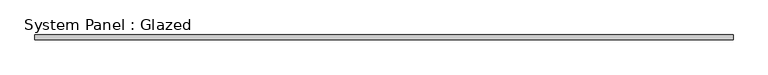
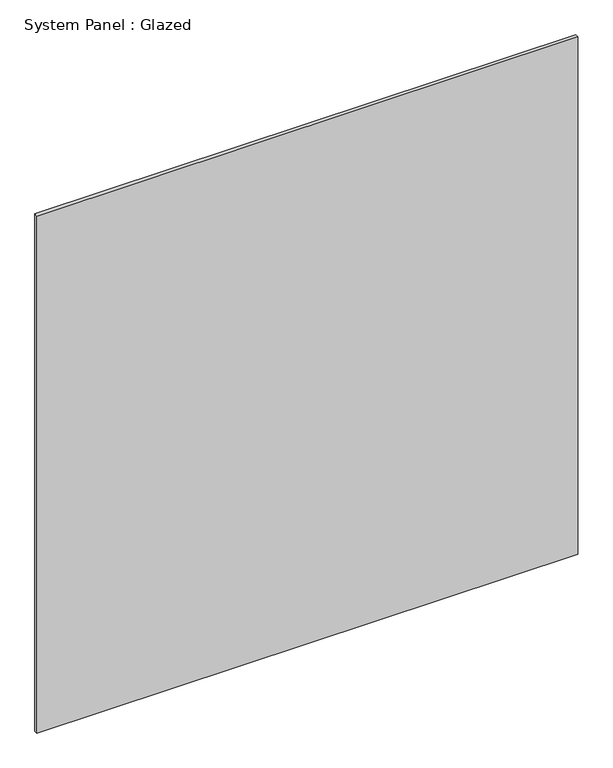
"""IFC4 building model written with IfcOpenShell, lengths in millimetres: plate geometry, System Panel : Glazed."""

from ifc_helpers import new_model, si_unit, origin, origin_with_axes, place, context, project, spatial, polyline, outline, extrude, source, transform, mapped, element, save


def system_panel_glazed_319e86f2(model_context):
    return source(origin(), model_context, "Body", "SweptSolid", [
        extrude(outline(polyline([(1896.6913473, 19.05), (-1896.6913473, 19.05), (-1896.6913473, 44.45), (1896.6913473, 44.45), (1896.6913473, 19.05)])), origin_with_axes(), (0.0, 0.0, 1.0), 3835.4),
    ])


if __name__ == "__main__":
    model = new_model("IFC4")
    model_context = context("Model", 3, world=origin())
    ifc_project = project(units=[si_unit("LENGTHUNIT", "METRE", prefix="MILLI")], contexts=[model_context])
    site = spatial("IfcSite", under=ifc_project)
    building = spatial("IfcBuilding", under=site)
    placement = place(None, origin())
    system_panel_glazed_shape = system_panel_glazed_319e86f2(model_context)
    element("IfcPlate", 1, ObjectType="System Panel : Glazed", at=placement, inside=building, context=model_context, shape_type="MappedRepresentation", body=[
        mapped(system_panel_glazed_shape, transform((0.0, 0.0, 0.0), x_axis=(1.0, 0.0, 0.0), y_axis=(0.0, 1.0, 0.0), z_axis=(0.0, 0.0, 1.0))),
    ])
    save(model, "model.ifc")

# Revit data of these elements
# Type "System Panel : Glazed"
#   Construction Type Id = "GSP4R"
#   Analytic Construction = "1/8 in Pilkington single glazing"
#   Visual Light Transmittance = 0.9
#   Solar Heat Gain Coefficient = 0.86
#   Heat Transfer Coefficient (U) = 1.18115 BTU/(h·ft²·°F)
# Element 1 (IfcPlate, "System Panel : Glazed")
#   Materials on its faces: "Glass"
# Materials
#   "Glass": class "Glass", colour RGB 0 128 192, transparency 0.75, Description = "Soda Lime Glass", Cost = 0
